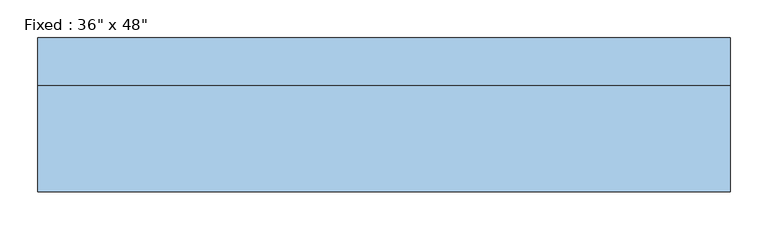
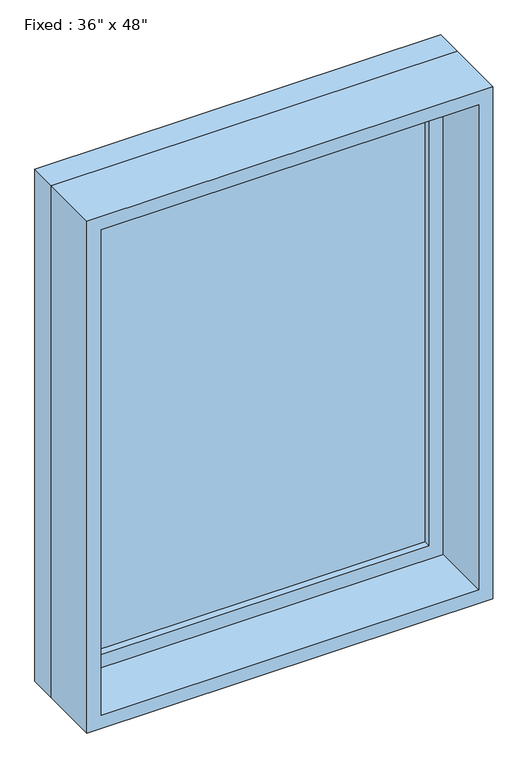
"""IFC4 building model written with IfcOpenShell, lengths in millimetres: window geometry."""

from ifc_helpers import new_model, si_unit, frame, origin, place, context, project, spatial, polyline, outline, extrude, source, transform, mapped, element, save


def window_e2841890(model_context):
    return source(origin(), model_context, "Body", "SweptSolid", [
        extrude(outline(polyline([(355.6, 53.975), (-431.8, 53.975), (-431.8, 66.675), (355.6, 66.675), (355.6, 53.975)])), frame((0.0, 0.0, 977.9), z_axis=(0.0, 0.0, 1.0), x_axis=(1.0, 0.0, 0.0)), (0.0, 0.0, 1.0), 1092.2),
        extrude(outline(polyline([(2114.55, -476.25), (933.45, -476.25), (933.45, 400.05), (2114.55, 400.05), (2114.55, -476.25)]), holes=[polyline([(2070.1, -431.8), (2070.1, 355.6), (977.9, 355.6), (977.9, -431.8), (2070.1, -431.8)])]), frame((0.0, 38.1, 0.0), z_axis=(0.0, 1.0, 0.0), x_axis=(0.0, 0.0, 1.0)), (0.0, 0.0, 1.0), 44.45),
        extrude(outline(polyline([(2133.6, -495.3), (914.4, -495.3), (914.4, 419.1), (2133.6, 419.1), (2133.6, -495.3)]), holes=[polyline([(2101.85, -463.55), (2101.85, 387.35), (946.15, 387.35), (946.15, -463.55), (2101.85, -463.55)])]), frame((0.0, -101.6, 0.0), z_axis=(0.0, 1.0, 0.0), x_axis=(0.0, 0.0, 1.0)), (0.0, 0.0, 1.0), 139.7),
        extrude(outline(polyline([(2133.6, 419.1), (2133.6, -495.3), (914.4, -495.3), (914.4, 419.1), (2133.6, 419.1)]), holes=[polyline([(2114.55, 400.05), (933.45, 400.05), (933.45, -476.25), (2114.55, -476.25), (2114.55, 400.05)])]), frame((0.0, 38.1, 0.0), z_axis=(0.0, 1.0, 0.0), x_axis=(0.0, 0.0, 1.0)), (0.0, 0.0, 1.0), 63.5),
    ])


if __name__ == "__main__":
    model = new_model("IFC4")
    model_context = context("Model", 3, world=origin())
    ifc_project = project(units=[si_unit("LENGTHUNIT", "METRE", prefix="MILLI")], contexts=[model_context])
    site = spatial("IfcSite", under=ifc_project)
    building = spatial("IfcBuilding", under=site)
    placement = place(None, origin())
    window_shape = window_e2841890(model_context)
    element("IfcWindow", 1, ObjectType="Fixed : 36\" x 48\"", at=placement, inside=building, context=model_context, shape_type="MappedRepresentation", body=[
        mapped(window_shape, transform((0.0, 0.0, 0.0), x_axis=(1.0, 0.0, 0.0), y_axis=(0.0, 1.0, 0.0), z_axis=(0.0, 0.0, 1.0))),
    ])
    save(model, "model.ifc")

# Revit data of these elements
# Type "Fixed : 36\" x 48\""
#   Type Mark = "1"
#   Assembly Code = "B2020100"
#   Height = 4' - 0"
#   Default Sill Height = 3' - 0"
#   Width = 3' - 0"
#   Window Inset = 0' - 0 3/4"
#   Glass Pane Material = Glass
#   Sash Material = Sash
#   Wall Closure = (empty or 0)
# Element 1 (IfcWindow, "Fixed : 36\" x 48\"")
#   Materials on its faces: "Sash", "Glass"
# Materials
#   "Glass": class "Glass", colour RGB 218 227 224, transparency 0.85, Description = "Soda Lime Glass", Cost = 0
#   "Sash": class "Wood", colour RGB 136 99 55, transparency 0
